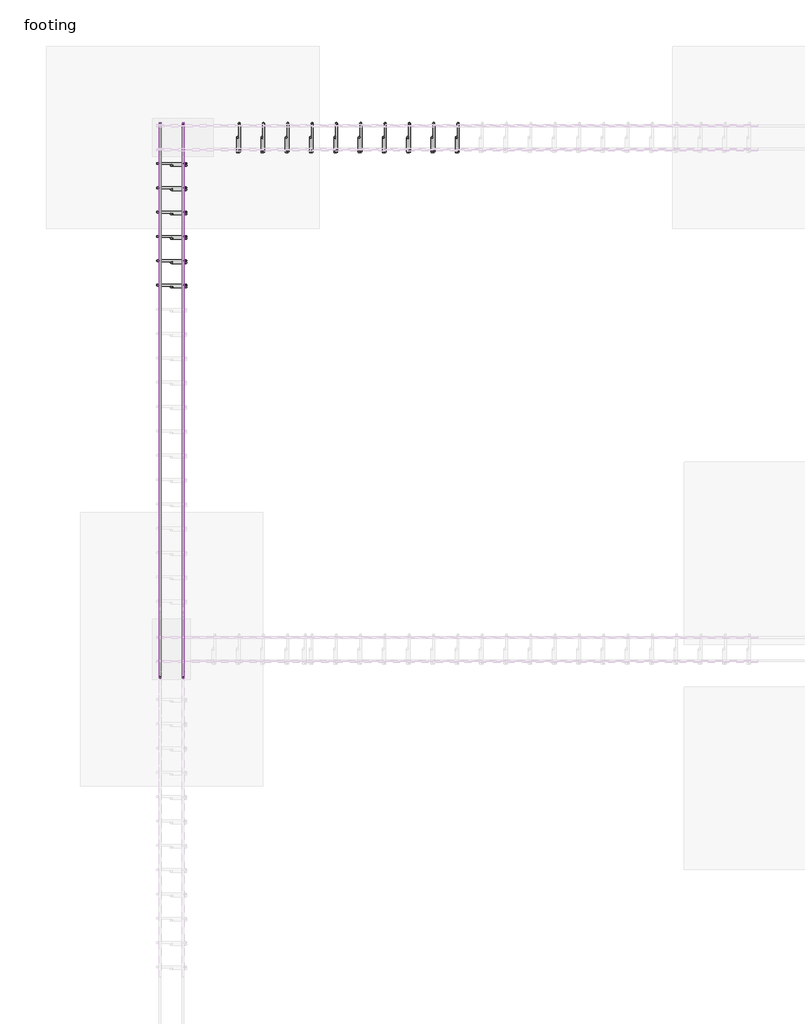
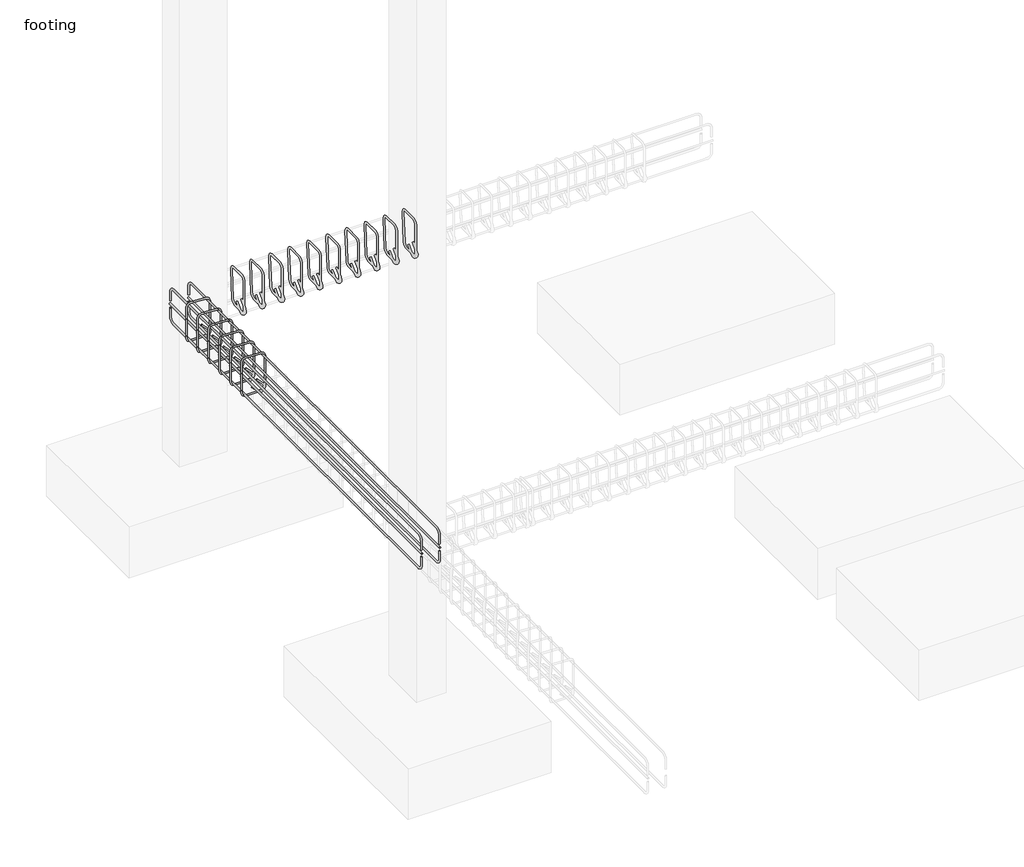
# One storey, part 16 of 21: 23 reinforcing bars.
"""IFC4 building model written with IfcOpenShell, lengths in millimetres."""

from ifc_helpers import new_model, si_unit, point, frame, origin, place, context, project, spatial, polyline, circle_curve, trimmed, segment, composite_curve, element, save
from ifc_brep_helpers import swept_disk

model = new_model("IFC4")

# Units and contexts
model_context = context("Model", 3, world=origin())
ifc_project = project(units=[si_unit("LENGTHUNIT", "METRE", prefix="MILLI")], contexts=[model_context])

# Site, building, storey
site = spatial("IfcSite", under=ifc_project)
building = spatial("IfcBuilding", under=site)
storey = spatial("IfcBuildingStorey", under=building, Name="footing", Elevation=-1524.0)

# Reinforcing bars
placement = place(None, origin())
element("IfcReinforcingBar", 1, at=placement, inside=storey, context=model_context, shape_type="SolidModel", body=[
    swept_disk(composite_curve([segment(polyline([(-11769.5883428, 10994.9387132, -310.8825168), (-11769.5883428, 10940.0737147, -365.7475153)]), True, "CONTINUOUS"), segment(trimmed(circle_curve(frame((-11769.5883428, 10917.6230744, -343.296875), z_axis=(-1.0, 0.0, 0.0), x_axis=(0.0, 22.450640299999577, -22.450640299999975)), 31.75), [point((-11769.5883428, 10940.0737147, -365.7475153))], [point((-11769.5883428, 10885.8730744, -343.296875))], True, "CARTESIAN"), True, "CONTINUOUS"), segment(polyline([(-11769.5883428, 10885.8730744, -343.296875), (-11769.5883428, 10885.8730744, -63.103125)]), True, "CONTINUOUS"), segment(trimmed(circle_curve(frame((-11769.5883428, 10917.6230744, -63.103125), z_axis=(-1.0, 0.0, 0.0), x_axis=(0.0, -31.75, 0.0)), 31.75), [point((-11769.5883428, 10885.8730744, -63.103125))], [point((-11769.5883428, 10917.6230744, -31.353125))], True, "CARTESIAN"), True, "CONTINUOUS"), segment(polyline([(-11769.5883428, 10917.6230744, -31.353125), (-11769.5883428, 11045.4168244, -31.353125)]), True, "CONTINUOUS"), segment(trimmed(circle_curve(frame((-11768.4159328, 11045.4168244, -63.0814712), z_axis=(-0.9993179916193466, 0.0, -0.03692629992126919), x_axis=(-1.1724099999992177, 0.0, 31.728346200000004)), 31.75), [point((-11769.5883428, 11045.4168244, -31.353125))], [point((-11768.4159328, 11077.1668244, -63.0814712))], True, "CARTESIAN"), True, "CONTINUOUS"), segment(polyline([(-11768.4159328, 11077.1668244, -63.0814712), (-11758.0607528, 11077.1668244, -343.3185288)]), True, "CONTINUOUS"), segment(trimmed(circle_curve(frame((-11758.0607528, 11045.4168244, -343.3185288), z_axis=(-0.9993179916193466, 0.0, -0.03692629992126919), x_axis=(0.0, 31.75, 0.0)), 31.75), [point((-11758.0607528, 11077.1668244, -343.3185288))], [point((-11756.8883428, 11045.4168244, -375.046875))], True, "CARTESIAN"), True, "CONTINUOUS"), segment(polyline([(-11756.8883428, 11045.4168244, -375.046875), (-11756.8883428, 10917.6230744, -375.046875)]), True, "CONTINUOUS"), segment(trimmed(circle_curve(frame((-11756.8883428, 10917.6230744, -343.296875), z_axis=(-1.0, 0.0, 0.0), x_axis=(0.0, 0.0, -31.75)), 31.75), [point((-11756.8883428, 10917.6230744, -375.046875))], [point((-11756.8883428, 10895.1724341, -320.8462347))], True, "CARTESIAN"), True, "CONTINUOUS"), segment(polyline([(-11756.8883428, 10895.1724341, -320.8462347), (-11756.8883428, 10950.0374326, -265.9812362)]), True, "CONTINUOUS")], self_intersect=False), 6.35),
])
element("IfcReinforcingBar", 2, at=placement, inside=storey, context=model_context, shape_type="SolidModel", body=[
    swept_disk(composite_curve([segment(polyline([(-11606.8883428, 10994.9387132, -310.8825168), (-11606.8883428, 10940.0737147, -365.7475153)]), True, "CONTINUOUS"), segment(trimmed(circle_curve(frame((-11606.8883428, 10917.6230744, -343.296875), z_axis=(-1.0, 0.0, 0.0), x_axis=(0.0, 22.450640299999577, -22.450640299999975)), 31.75), [point((-11606.8883428, 10940.0737147, -365.7475153))], [point((-11606.8883428, 10885.8730744, -343.296875))], True, "CARTESIAN"), True, "CONTINUOUS"), segment(polyline([(-11606.8883428, 10885.8730744, -343.296875), (-11606.8883428, 10885.8730744, -63.103125)]), True, "CONTINUOUS"), segment(trimmed(circle_curve(frame((-11606.8883428, 10917.6230744, -63.103125), z_axis=(-1.0, 0.0, 0.0), x_axis=(0.0, -31.75, 0.0)), 31.75), [point((-11606.8883428, 10885.8730744, -63.103125))], [point((-11606.8883428, 10917.6230744, -31.353125))], True, "CARTESIAN"), True, "CONTINUOUS"), segment(polyline([(-11606.8883428, 10917.6230744, -31.353125), (-11606.8883428, 11045.4168244, -31.353125)]), True, "CONTINUOUS"), segment(trimmed(circle_curve(frame((-11605.7159328, 11045.4168244, -63.0814712), z_axis=(-0.9993179916193466, 0.0, -0.03692629992126919), x_axis=(-1.1724100000010367, 0.0, 31.728346200000004)), 31.75), [point((-11606.8883428, 11045.4168244, -31.353125))], [point((-11605.7159328, 11077.1668244, -63.0814712))], True, "CARTESIAN"), True, "CONTINUOUS"), segment(polyline([(-11605.7159328, 11077.1668244, -63.0814712), (-11595.3607528, 11077.1668244, -343.3185288)]), True, "CONTINUOUS"), segment(trimmed(circle_curve(frame((-11595.3607528, 11045.4168244, -343.3185288), z_axis=(-0.9993179916193466, 0.0, -0.03692629992126919), x_axis=(0.0, 31.75, 0.0)), 31.75), [point((-11595.3607528, 11077.1668244, -343.3185288))], [point((-11594.1883428, 11045.4168244, -375.046875))], True, "CARTESIAN"), True, "CONTINUOUS"), segment(polyline([(-11594.1883428, 11045.4168244, -375.046875), (-11594.1883428, 10917.6230744, -375.046875)]), True, "CONTINUOUS"), segment(trimmed(circle_curve(frame((-11594.1883428, 10917.6230744, -343.296875), z_axis=(-1.0, 0.0, 0.0), x_axis=(0.0, 0.0, -31.75)), 31.75), [point((-11594.1883428, 10917.6230744, -375.046875))], [point((-11594.1883428, 10895.1724341, -320.8462347))], True, "CARTESIAN"), True, "CONTINUOUS"), segment(polyline([(-11594.1883428, 10895.1724341, -320.8462347), (-11594.1883428, 10950.0374326, -265.9812362)]), True, "CONTINUOUS")], self_intersect=False), 6.35),
])
element("IfcReinforcingBar", 3, at=placement, inside=storey, context=model_context, shape_type="SolidModel", body=[
    swept_disk(composite_curve([segment(polyline([(-11444.1883428, 10994.9387132, -310.8825168), (-11444.1883428, 10940.0737147, -365.7475153)]), True, "CONTINUOUS"), segment(trimmed(circle_curve(frame((-11444.1883428, 10917.6230744, -343.296875), z_axis=(-1.0, 0.0, 0.0), x_axis=(0.0, 22.450640299999577, -22.450640299999975)), 31.75), [point((-11444.1883428, 10940.0737147, -365.7475153))], [point((-11444.1883428, 10885.8730744, -343.296875))], True, "CARTESIAN"), True, "CONTINUOUS"), segment(polyline([(-11444.1883428, 10885.8730744, -343.296875), (-11444.1883428, 10885.8730744, -63.103125)]), True, "CONTINUOUS"), segment(trimmed(circle_curve(frame((-11444.1883428, 10917.6230744, -63.103125), z_axis=(-1.0, 0.0, 0.0), x_axis=(0.0, -31.75, 0.0)), 31.75), [point((-11444.1883428, 10885.8730744, -63.103125))], [point((-11444.1883428, 10917.6230744, -31.353125))], True, "CARTESIAN"), True, "CONTINUOUS"), segment(polyline([(-11444.1883428, 10917.6230744, -31.353125), (-11444.1883428, 11045.4168244, -31.353125)]), True, "CONTINUOUS"), segment(trimmed(circle_curve(frame((-11443.0159328, 11045.4168244, -63.0814712), z_axis=(-0.9993179916193466, 0.0, -0.03692629992126919), x_axis=(-1.1724099999992177, 0.0, 31.728346200000004)), 31.75), [point((-11444.1883428, 11045.4168244, -31.353125))], [point((-11443.0159328, 11077.1668244, -63.0814712))], True, "CARTESIAN"), True, "CONTINUOUS"), segment(polyline([(-11443.0159328, 11077.1668244, -63.0814712), (-11432.6607528, 11077.1668244, -343.3185288)]), True, "CONTINUOUS"), segment(trimmed(circle_curve(frame((-11432.6607528, 11045.4168244, -343.3185288), z_axis=(-0.9993179916193466, 0.0, -0.03692629992126919), x_axis=(0.0, 31.75, 0.0)), 31.75), [point((-11432.6607528, 11077.1668244, -343.3185288))], [point((-11431.4883428, 11045.4168244, -375.046875))], True, "CARTESIAN"), True, "CONTINUOUS"), segment(polyline([(-11431.4883428, 11045.4168244, -375.046875), (-11431.4883428, 10917.6230744, -375.046875)]), True, "CONTINUOUS"), segment(trimmed(circle_curve(frame((-11431.4883428, 10917.6230744, -343.296875), z_axis=(-1.0, 0.0, 0.0), x_axis=(0.0, 0.0, -31.75)), 31.75), [point((-11431.4883428, 10917.6230744, -375.046875))], [point((-11431.4883428, 10895.1724341, -320.8462347))], True, "CARTESIAN"), True, "CONTINUOUS"), segment(polyline([(-11431.4883428, 10895.1724341, -320.8462347), (-11431.4883428, 10950.0374326, -265.9812362)]), True, "CONTINUOUS")], self_intersect=False), 6.35),
])
element("IfcReinforcingBar", 4, at=placement, inside=storey, context=model_context, shape_type="SolidModel", body=[
    swept_disk(composite_curve([segment(polyline([(-11281.4883428, 10994.9387132, -310.8825168), (-11281.4883428, 10940.0737147, -365.7475153)]), True, "CONTINUOUS"), segment(trimmed(circle_curve(frame((-11281.4883428, 10917.6230744, -343.296875), z_axis=(-1.0, 0.0, 0.0), x_axis=(0.0, 22.450640299999577, -22.450640299999975)), 31.75), [point((-11281.4883428, 10940.0737147, -365.7475153))], [point((-11281.4883428, 10885.8730744, -343.296875))], True, "CARTESIAN"), True, "CONTINUOUS"), segment(polyline([(-11281.4883428, 10885.8730744, -343.296875), (-11281.4883428, 10885.8730744, -63.103125)]), True, "CONTINUOUS"), segment(trimmed(circle_curve(frame((-11281.4883428, 10917.6230744, -63.103125), z_axis=(-1.0, 0.0, 0.0), x_axis=(0.0, -31.75, 0.0)), 31.75), [point((-11281.4883428, 10885.8730744, -63.103125))], [point((-11281.4883428, 10917.6230744, -31.353125))], True, "CARTESIAN"), True, "CONTINUOUS"), segment(polyline([(-11281.4883428, 10917.6230744, -31.353125), (-11281.4883428, 11045.4168244, -31.353125)]), True, "CONTINUOUS"), segment(trimmed(circle_curve(frame((-11280.3159328, 11045.4168244, -63.0814712), z_axis=(-0.9993179916193466, 0.0, -0.03692629992126919), x_axis=(-1.1724099999992177, 0.0, 31.728346200000004)), 31.75), [point((-11281.4883428, 11045.4168244, -31.353125))], [point((-11280.3159328, 11077.1668244, -63.0814712))], True, "CARTESIAN"), True, "CONTINUOUS"), segment(polyline([(-11280.3159328, 11077.1668244, -63.0814712), (-11269.9607528, 11077.1668244, -343.3185288)]), True, "CONTINUOUS"), segment(trimmed(circle_curve(frame((-11269.9607528, 11045.4168244, -343.3185288), z_axis=(-0.9993179916193466, 0.0, -0.03692629992126919), x_axis=(0.0, 31.75, 0.0)), 31.75), [point((-11269.9607528, 11077.1668244, -343.3185288))], [point((-11268.7883428, 11045.4168244, -375.046875))], True, "CARTESIAN"), True, "CONTINUOUS"), segment(polyline([(-11268.7883428, 11045.4168244, -375.046875), (-11268.7883428, 10917.6230744, -375.046875)]), True, "CONTINUOUS"), segment(trimmed(circle_curve(frame((-11268.7883428, 10917.6230744, -343.296875), z_axis=(-1.0, 0.0, 0.0), x_axis=(0.0, 0.0, -31.75)), 31.75), [point((-11268.7883428, 10917.6230744, -375.046875))], [point((-11268.7883428, 10895.1724341, -320.8462347))], True, "CARTESIAN"), True, "CONTINUOUS"), segment(polyline([(-11268.7883428, 10895.1724341, -320.8462347), (-11268.7883428, 10950.0374326, -265.9812362)]), True, "CONTINUOUS")], self_intersect=False), 6.35),
])
element("IfcReinforcingBar", 5, at=placement, inside=storey, context=model_context, shape_type="SolidModel", body=[
    swept_disk(composite_curve([segment(polyline([(-11118.7883428, 10994.9387132, -310.8825168), (-11118.7883428, 10940.0737147, -365.7475153)]), True, "CONTINUOUS"), segment(trimmed(circle_curve(frame((-11118.7883428, 10917.6230744, -343.296875), z_axis=(-1.0, 0.0, 0.0), x_axis=(0.0, 22.450640299999577, -22.450640299999975)), 31.75), [point((-11118.7883428, 10940.0737147, -365.7475153))], [point((-11118.7883428, 10885.8730744, -343.296875))], True, "CARTESIAN"), True, "CONTINUOUS"), segment(polyline([(-11118.7883428, 10885.8730744, -343.296875), (-11118.7883428, 10885.8730744, -63.103125)]), True, "CONTINUOUS"), segment(trimmed(circle_curve(frame((-11118.7883428, 10917.6230744, -63.103125), z_axis=(-1.0, 0.0, 0.0), x_axis=(0.0, -31.75, 0.0)), 31.75), [point((-11118.7883428, 10885.8730744, -63.103125))], [point((-11118.7883428, 10917.6230744, -31.353125))], True, "CARTESIAN"), True, "CONTINUOUS"), segment(polyline([(-11118.7883428, 10917.6230744, -31.353125), (-11118.7883428, 11045.4168244, -31.353125)]), True, "CONTINUOUS"), segment(trimmed(circle_curve(frame((-11117.6159328, 11045.4168244, -63.0814712), z_axis=(-0.9993179916193466, 0.0, -0.03692629992126919), x_axis=(-1.1724100000010367, 0.0, 31.728346200000004)), 31.75), [point((-11118.7883428, 11045.4168244, -31.353125))], [point((-11117.6159328, 11077.1668244, -63.0814712))], True, "CARTESIAN"), True, "CONTINUOUS"), segment(polyline([(-11117.6159328, 11077.1668244, -63.0814712), (-11107.2607528, 11077.1668244, -343.3185288)]), True, "CONTINUOUS"), segment(trimmed(circle_curve(frame((-11107.2607528, 11045.4168244, -343.3185288), z_axis=(-0.9993179916193466, 0.0, -0.03692629992126919), x_axis=(0.0, 31.75, 0.0)), 31.75), [point((-11107.2607528, 11077.1668244, -343.3185288))], [point((-11106.0883428, 11045.4168244, -375.046875))], True, "CARTESIAN"), True, "CONTINUOUS"), segment(polyline([(-11106.0883428, 11045.4168244, -375.046875), (-11106.0883428, 10917.6230744, -375.046875)]), True, "CONTINUOUS"), segment(trimmed(circle_curve(frame((-11106.0883428, 10917.6230744, -343.296875), z_axis=(-1.0, 0.0, 0.0), x_axis=(0.0, 0.0, -31.75)), 31.75), [point((-11106.0883428, 10917.6230744, -375.046875))], [point((-11106.0883428, 10895.1724341, -320.8462347))], True, "CARTESIAN"), True, "CONTINUOUS"), segment(polyline([(-11106.0883428, 10895.1724341, -320.8462347), (-11106.0883428, 10950.0374326, -265.9812362)]), True, "CONTINUOUS")], self_intersect=False), 6.35),
])
element("IfcReinforcingBar", 6, at=placement, inside=storey, context=model_context, shape_type="SolidModel", body=[
    swept_disk(composite_curve([segment(polyline([(-10956.0883428, 10994.9387132, -310.8825168), (-10956.0883428, 10940.0737147, -365.7475153)]), True, "CONTINUOUS"), segment(trimmed(circle_curve(frame((-10956.0883428, 10917.6230744, -343.296875), z_axis=(-1.0, 0.0, 0.0), x_axis=(0.0, 22.450640299999577, -22.450640299999975)), 31.75), [point((-10956.0883428, 10940.0737147, -365.7475153))], [point((-10956.0883428, 10885.8730744, -343.296875))], True, "CARTESIAN"), True, "CONTINUOUS"), segment(polyline([(-10956.0883428, 10885.8730744, -343.296875), (-10956.0883428, 10885.8730744, -63.103125)]), True, "CONTINUOUS"), segment(trimmed(circle_curve(frame((-10956.0883428, 10917.6230744, -63.103125), z_axis=(-1.0, 0.0, 0.0), x_axis=(0.0, -31.75, 0.0)), 31.75), [point((-10956.0883428, 10885.8730744, -63.103125))], [point((-10956.0883428, 10917.6230744, -31.353125))], True, "CARTESIAN"), True, "CONTINUOUS"), segment(polyline([(-10956.0883428, 10917.6230744, -31.353125), (-10956.0883428, 11045.4168244, -31.353125)]), True, "CONTINUOUS"), segment(trimmed(circle_curve(frame((-10954.9159328, 11045.4168244, -63.0814712), z_axis=(-0.9993179916193466, 0.0, -0.03692629992126919), x_axis=(-1.1724099999992177, 0.0, 31.728346200000004)), 31.75), [point((-10956.0883428, 11045.4168244, -31.353125))], [point((-10954.9159328, 11077.1668244, -63.0814712))], True, "CARTESIAN"), True, "CONTINUOUS"), segment(polyline([(-10954.9159328, 11077.1668244, -63.0814712), (-10944.5607528, 11077.1668244, -343.3185288)]), True, "CONTINUOUS"), segment(trimmed(circle_curve(frame((-10944.5607528, 11045.4168244, -343.3185288), z_axis=(-0.9993179916193466, 0.0, -0.03692629992126919), x_axis=(0.0, 31.75, 0.0)), 31.75), [point((-10944.5607528, 11077.1668244, -343.3185288))], [point((-10943.3883428, 11045.4168244, -375.046875))], True, "CARTESIAN"), True, "CONTINUOUS"), segment(polyline([(-10943.3883428, 11045.4168244, -375.046875), (-10943.3883428, 10917.6230744, -375.046875)]), True, "CONTINUOUS"), segment(trimmed(circle_curve(frame((-10943.3883428, 10917.6230744, -343.296875), z_axis=(-1.0, 0.0, 0.0), x_axis=(0.0, 0.0, -31.75)), 31.75), [point((-10943.3883428, 10917.6230744, -375.046875))], [point((-10943.3883428, 10895.1724341, -320.8462347))], True, "CARTESIAN"), True, "CONTINUOUS"), segment(polyline([(-10943.3883428, 10895.1724341, -320.8462347), (-10943.3883428, 10950.0374326, -265.9812362)]), True, "CONTINUOUS")], self_intersect=False), 6.35),
])
element("IfcReinforcingBar", 7, at=placement, inside=storey, context=model_context, shape_type="SolidModel", body=[
    swept_disk(composite_curve([segment(polyline([(-10793.3883428, 10994.9387132, -310.8825168), (-10793.3883428, 10940.0737147, -365.7475153)]), True, "CONTINUOUS"), segment(trimmed(circle_curve(frame((-10793.3883428, 10917.6230744, -343.296875), z_axis=(-1.0, 0.0, 0.0), x_axis=(0.0, 22.450640299999577, -22.450640299999975)), 31.75), [point((-10793.3883428, 10940.0737147, -365.7475153))], [point((-10793.3883428, 10885.8730744, -343.296875))], True, "CARTESIAN"), True, "CONTINUOUS"), segment(polyline([(-10793.3883428, 10885.8730744, -343.296875), (-10793.3883428, 10885.8730744, -63.103125)]), True, "CONTINUOUS"), segment(trimmed(circle_curve(frame((-10793.3883428, 10917.6230744, -63.103125), z_axis=(-1.0, 0.0, 0.0), x_axis=(0.0, -31.75, 0.0)), 31.75), [point((-10793.3883428, 10885.8730744, -63.103125))], [point((-10793.3883428, 10917.6230744, -31.353125))], True, "CARTESIAN"), True, "CONTINUOUS"), segment(polyline([(-10793.3883428, 10917.6230744, -31.353125), (-10793.3883428, 11045.4168244, -31.353125)]), True, "CONTINUOUS"), segment(trimmed(circle_curve(frame((-10792.2159328, 11045.4168244, -63.0814712), z_axis=(-0.9993179916193466, 0.0, -0.03692629992126919), x_axis=(-1.1724100000010367, 0.0, 31.728346200000004)), 31.75), [point((-10793.3883428, 11045.4168244, -31.353125))], [point((-10792.2159328, 11077.1668244, -63.0814712))], True, "CARTESIAN"), True, "CONTINUOUS"), segment(polyline([(-10792.2159328, 11077.1668244, -63.0814712), (-10781.8607528, 11077.1668244, -343.3185288)]), True, "CONTINUOUS"), segment(trimmed(circle_curve(frame((-10781.8607528, 11045.4168244, -343.3185288), z_axis=(-0.9993179916193466, 0.0, -0.03692629992126919), x_axis=(0.0, 31.75, 0.0)), 31.75), [point((-10781.8607528, 11077.1668244, -343.3185288))], [point((-10780.6883428, 11045.4168244, -375.046875))], True, "CARTESIAN"), True, "CONTINUOUS"), segment(polyline([(-10780.6883428, 11045.4168244, -375.046875), (-10780.6883428, 10917.6230744, -375.046875)]), True, "CONTINUOUS"), segment(trimmed(circle_curve(frame((-10780.6883428, 10917.6230744, -343.296875), z_axis=(-1.0, 0.0, 0.0), x_axis=(0.0, 0.0, -31.75)), 31.75), [point((-10780.6883428, 10917.6230744, -375.046875))], [point((-10780.6883428, 10895.1724341, -320.8462347))], True, "CARTESIAN"), True, "CONTINUOUS"), segment(polyline([(-10780.6883428, 10895.1724341, -320.8462347), (-10780.6883428, 10950.0374326, -265.9812362)]), True, "CONTINUOUS")], self_intersect=False), 6.35),
])
element("IfcReinforcingBar", 8, at=placement, inside=storey, context=model_context, shape_type="SolidModel", body=[
    swept_disk(composite_curve([segment(polyline([(-10630.6883428, 10994.9387132, -310.8825168), (-10630.6883428, 10940.0737147, -365.7475153)]), True, "CONTINUOUS"), segment(trimmed(circle_curve(frame((-10630.6883428, 10917.6230744, -343.296875), z_axis=(-1.0, 0.0, 0.0), x_axis=(0.0, 22.450640299999577, -22.450640299999975)), 31.75), [point((-10630.6883428, 10940.0737147, -365.7475153))], [point((-10630.6883428, 10885.8730744, -343.296875))], True, "CARTESIAN"), True, "CONTINUOUS"), segment(polyline([(-10630.6883428, 10885.8730744, -343.296875), (-10630.6883428, 10885.8730744, -63.103125)]), True, "CONTINUOUS"), segment(trimmed(circle_curve(frame((-10630.6883428, 10917.6230744, -63.103125), z_axis=(-1.0, 0.0, 0.0), x_axis=(0.0, -31.75, 0.0)), 31.75), [point((-10630.6883428, 10885.8730744, -63.103125))], [point((-10630.6883428, 10917.6230744, -31.353125))], True, "CARTESIAN"), True, "CONTINUOUS"), segment(polyline([(-10630.6883428, 10917.6230744, -31.353125), (-10630.6883428, 11045.4168244, -31.353125)]), True, "CONTINUOUS"), segment(trimmed(circle_curve(frame((-10629.5159328, 11045.4168244, -63.0814712), z_axis=(-0.9993179916193466, 0.0, -0.03692629992126919), x_axis=(-1.1724099999992177, 0.0, 31.728346200000004)), 31.75), [point((-10630.6883428, 11045.4168244, -31.353125))], [point((-10629.5159328, 11077.1668244, -63.0814712))], True, "CARTESIAN"), True, "CONTINUOUS"), segment(polyline([(-10629.5159328, 11077.1668244, -63.0814712), (-10619.1607528, 11077.1668244, -343.3185288)]), True, "CONTINUOUS"), segment(trimmed(circle_curve(frame((-10619.1607528, 11045.4168244, -343.3185288), z_axis=(-0.9993179916193466, 0.0, -0.03692629992126919), x_axis=(0.0, 31.75, 0.0)), 31.75), [point((-10619.1607528, 11077.1668244, -343.3185288))], [point((-10617.9883428, 11045.4168244, -375.046875))], True, "CARTESIAN"), True, "CONTINUOUS"), segment(polyline([(-10617.9883428, 11045.4168244, -375.046875), (-10617.9883428, 10917.6230744, -375.046875)]), True, "CONTINUOUS"), segment(trimmed(circle_curve(frame((-10617.9883428, 10917.6230744, -343.296875), z_axis=(-1.0, 0.0, 0.0), x_axis=(0.0, 0.0, -31.75)), 31.75), [point((-10617.9883428, 10917.6230744, -375.046875))], [point((-10617.9883428, 10895.1724341, -320.8462347))], True, "CARTESIAN"), True, "CONTINUOUS"), segment(polyline([(-10617.9883428, 10895.1724341, -320.8462347), (-10617.9883428, 10950.0374326, -265.9812362)]), True, "CONTINUOUS")], self_intersect=False), 6.35),
])
element("IfcReinforcingBar", 9, at=placement, inside=storey, context=model_context, shape_type="SolidModel", body=[
    swept_disk(composite_curve([segment(polyline([(-10467.9883428, 10994.9387132, -310.8825168), (-10467.9883428, 10940.0737147, -365.7475153)]), True, "CONTINUOUS"), segment(trimmed(circle_curve(frame((-10467.9883428, 10917.6230744, -343.296875), z_axis=(-1.0, 0.0, 0.0), x_axis=(0.0, 22.450640299999577, -22.450640299999975)), 31.75), [point((-10467.9883428, 10940.0737147, -365.7475153))], [point((-10467.9883428, 10885.8730744, -343.296875))], True, "CARTESIAN"), True, "CONTINUOUS"), segment(polyline([(-10467.9883428, 10885.8730744, -343.296875), (-10467.9883428, 10885.8730744, -63.103125)]), True, "CONTINUOUS"), segment(trimmed(circle_curve(frame((-10467.9883428, 10917.6230744, -63.103125), z_axis=(-1.0, 0.0, 0.0), x_axis=(0.0, -31.75, 0.0)), 31.75), [point((-10467.9883428, 10885.8730744, -63.103125))], [point((-10467.9883428, 10917.6230744, -31.353125))], True, "CARTESIAN"), True, "CONTINUOUS"), segment(polyline([(-10467.9883428, 10917.6230744, -31.353125), (-10467.9883428, 11045.4168244, -31.353125)]), True, "CONTINUOUS"), segment(trimmed(circle_curve(frame((-10466.8159328, 11045.4168244, -63.0814712), z_axis=(-0.9993179916193466, 0.0, -0.03692629992126919), x_axis=(-1.1724099999992177, 0.0, 31.728346200000004)), 31.75), [point((-10467.9883428, 11045.4168244, -31.353125))], [point((-10466.8159328, 11077.1668244, -63.0814712))], True, "CARTESIAN"), True, "CONTINUOUS"), segment(polyline([(-10466.8159328, 11077.1668244, -63.0814712), (-10456.4607528, 11077.1668244, -343.3185288)]), True, "CONTINUOUS"), segment(trimmed(circle_curve(frame((-10456.4607528, 11045.4168244, -343.3185288), z_axis=(-0.9993179916193466, 0.0, -0.03692629992126919), x_axis=(0.0, 31.75, 0.0)), 31.75), [point((-10456.4607528, 11077.1668244, -343.3185288))], [point((-10455.2883428, 11045.4168244, -375.046875))], True, "CARTESIAN"), True, "CONTINUOUS"), segment(polyline([(-10455.2883428, 11045.4168244, -375.046875), (-10455.2883428, 10917.6230744, -375.046875)]), True, "CONTINUOUS"), segment(trimmed(circle_curve(frame((-10455.2883428, 10917.6230744, -343.296875), z_axis=(-1.0, 0.0, 0.0), x_axis=(0.0, 0.0, -31.75)), 31.75), [point((-10455.2883428, 10917.6230744, -375.046875))], [point((-10455.2883428, 10895.1724341, -320.8462347))], True, "CARTESIAN"), True, "CONTINUOUS"), segment(polyline([(-10455.2883428, 10895.1724341, -320.8462347), (-10455.2883428, 10950.0374326, -265.9812362)]), True, "CONTINUOUS")], self_intersect=False), 6.35),
])
element("IfcReinforcingBar", 10, at=placement, inside=storey, context=model_context, shape_type="SolidModel", body=[
    swept_disk(composite_curve([segment(polyline([(-10305.2883428, 10994.9387132, -310.8825168), (-10305.2883428, 10940.0737147, -365.7475153)]), True, "CONTINUOUS"), segment(trimmed(circle_curve(frame((-10305.2883428, 10917.6230744, -343.296875), z_axis=(-1.0, 0.0, 0.0), x_axis=(0.0, 22.450640299999577, -22.450640299999975)), 31.75), [point((-10305.2883428, 10940.0737147, -365.7475153))], [point((-10305.2883428, 10885.8730744, -343.296875))], True, "CARTESIAN"), True, "CONTINUOUS"), segment(polyline([(-10305.2883428, 10885.8730744, -343.296875), (-10305.2883428, 10885.8730744, -63.103125)]), True, "CONTINUOUS"), segment(trimmed(circle_curve(frame((-10305.2883428, 10917.6230744, -63.103125), z_axis=(-1.0, 0.0, 0.0), x_axis=(0.0, -31.75, 0.0)), 31.75), [point((-10305.2883428, 10885.8730744, -63.103125))], [point((-10305.2883428, 10917.6230744, -31.353125))], True, "CARTESIAN"), True, "CONTINUOUS"), segment(polyline([(-10305.2883428, 10917.6230744, -31.353125), (-10305.2883428, 11045.4168244, -31.353125)]), True, "CONTINUOUS"), segment(trimmed(circle_curve(frame((-10304.1159328, 11045.4168244, -63.0814712), z_axis=(-0.9993179916193466, 0.0, -0.03692629992126919), x_axis=(-1.1724100000010367, 0.0, 31.728346200000004)), 31.75), [point((-10305.2883428, 11045.4168244, -31.353125))], [point((-10304.1159328, 11077.1668244, -63.0814712))], True, "CARTESIAN"), True, "CONTINUOUS"), segment(polyline([(-10304.1159328, 11077.1668244, -63.0814712), (-10293.7607528, 11077.1668244, -343.3185288)]), True, "CONTINUOUS"), segment(trimmed(circle_curve(frame((-10293.7607528, 11045.4168244, -343.3185288), z_axis=(-0.9993179916193466, 0.0, -0.03692629992126919), x_axis=(0.0, 31.75, 0.0)), 31.75), [point((-10293.7607528, 11077.1668244, -343.3185288))], [point((-10292.5883428, 11045.4168244, -375.046875))], True, "CARTESIAN"), True, "CONTINUOUS"), segment(polyline([(-10292.5883428, 11045.4168244, -375.046875), (-10292.5883428, 10917.6230744, -375.046875)]), True, "CONTINUOUS"), segment(trimmed(circle_curve(frame((-10292.5883428, 10917.6230744, -343.296875), z_axis=(-1.0, 0.0, 0.0), x_axis=(0.0, 0.0, -31.75)), 31.75), [point((-10292.5883428, 10917.6230744, -375.046875))], [point((-10292.5883428, 10895.1724341, -320.8462347))], True, "CARTESIAN"), True, "CONTINUOUS"), segment(polyline([(-10292.5883428, 10895.1724341, -320.8462347), (-10292.5883428, 10950.0374326, -265.9812362)]), True, "CONTINUOUS")], self_intersect=False), 6.35),
])
element("IfcReinforcingBar", 11, at=placement, inside=storey, context=model_context, shape_type="SolidModel", body=[
    swept_disk(composite_curve([segment(polyline([(-12178.1165254, 9995.2456073, -265.9812362), (-12123.251527, 9995.2456073, -320.8462347)]), True, "CONTINUOUS"), segment(trimmed(circle_curve(frame((-12145.7021673, 9995.2456073, -343.296875), z_axis=(0.0, 1.0, 0.0), x_axis=(22.450640299999577, 0.0, 22.450640299999975)), 31.75), [point((-12123.251527, 9995.2456073, -320.8462347))], [point((-12145.7021673, 9995.2456073, -375.046875))], True, "CARTESIAN"), True, "CONTINUOUS"), segment(polyline([(-12145.7021673, 9995.2456073, -375.046875), (-12273.4959173, 9995.2456073, -375.046875)]), True, "CONTINUOUS"), segment(trimmed(circle_curve(frame((-12273.4959173, 9995.2456073, -343.296875), z_axis=(0.0, 1.0, 0.0), x_axis=(0.0, 0.0, -31.75)), 31.75), [point((-12273.4959173, 9995.2456073, -375.046875))], [point((-12305.2459173, 9995.2456073, -343.296875))], True, "CARTESIAN"), True, "CONTINUOUS"), segment(polyline([(-12305.2459173, 9995.2456073, -343.296875), (-12305.2459173, 9995.2456073, -63.103125)]), True, "CONTINUOUS"), segment(trimmed(circle_curve(frame((-12273.565658, 9993.1423536, -63.103125), z_axis=(0.0662442117686417, 0.9978034397651431, 0.0), x_axis=(-31.680259300001126, 2.103253699999186, 0.0)), 31.75), [point((-12305.2459173, 9995.2456073, -63.103125))], [point((-12273.565658, 9993.1423536, -31.353125))], True, "CARTESIAN"), True, "CONTINUOUS"), segment(polyline([(-12273.565658, 9993.1423536, -31.353125), (-12145.6324265, 9984.648861, -31.353125)]), True, "CONTINUOUS"), segment(trimmed(circle_curve(frame((-12145.6324265, 9984.648861, -63.103125), z_axis=(0.06624421176864169, 0.997803439765143, 0.0), x_axis=(0.0, 0.0, 31.75)), 31.75), [point((-12145.6324265, 9984.648861, -31.353125))], [point((-12113.9521673, 9982.5456073, -63.103125))], True, "CARTESIAN"), True, "CONTINUOUS"), segment(polyline([(-12113.9521673, 9982.5456073, -63.103125), (-12113.9521673, 9982.5456073, -343.296875)]), True, "CONTINUOUS"), segment(trimmed(circle_curve(frame((-12145.7021673, 9982.5456073, -343.296875), z_axis=(0.0, 1.0, 0.0), x_axis=(31.75, 0.0, 0.0)), 31.75), [point((-12113.9521673, 9982.5456073, -343.296875))], [point((-12168.1528076, 9982.5456073, -365.7475153))], True, "CARTESIAN"), True, "CONTINUOUS"), segment(polyline([(-12168.1528076, 9982.5456073, -365.7475153), (-12223.017806, 9982.5456073, -310.8825168)]), True, "CONTINUOUS")], self_intersect=False), 6.35),
])
element("IfcReinforcingBar", 12, at=placement, inside=storey, context=model_context, shape_type="SolidModel", body=[
    swept_disk(composite_curve([segment(polyline([(-12178.1165254, 10157.9456073, -265.9812362), (-12123.251527, 10157.9456073, -320.8462347)]), True, "CONTINUOUS"), segment(trimmed(circle_curve(frame((-12145.7021673, 10157.9456073, -343.296875), z_axis=(0.0, 1.0, 0.0), x_axis=(22.450640299999577, 0.0, 22.450640299999975)), 31.75), [point((-12123.251527, 10157.9456073, -320.8462347))], [point((-12145.7021673, 10157.9456073, -375.046875))], True, "CARTESIAN"), True, "CONTINUOUS"), segment(polyline([(-12145.7021673, 10157.9456073, -375.046875), (-12273.4959173, 10157.9456073, -375.046875)]), True, "CONTINUOUS"), segment(trimmed(circle_curve(frame((-12273.4959173, 10157.9456073, -343.296875), z_axis=(0.0, 1.0, 0.0), x_axis=(0.0, 0.0, -31.75)), 31.75), [point((-12273.4959173, 10157.9456073, -375.046875))], [point((-12305.2459173, 10157.9456073, -343.296875))], True, "CARTESIAN"), True, "CONTINUOUS"), segment(polyline([(-12305.2459173, 10157.9456073, -343.296875), (-12305.2459173, 10157.9456073, -63.103125)]), True, "CONTINUOUS"), segment(trimmed(circle_curve(frame((-12273.565658, 10155.8423536, -63.103125), z_axis=(0.0662442117686417, 0.9978034397651431, 0.0), x_axis=(-31.680259300001126, 2.103253700001005, 0.0)), 31.75), [point((-12305.2459173, 10157.9456073, -63.103125))], [point((-12273.565658, 10155.8423536, -31.353125))], True, "CARTESIAN"), True, "CONTINUOUS"), segment(polyline([(-12273.565658, 10155.8423536, -31.353125), (-12145.6324265, 10147.348861, -31.353125)]), True, "CONTINUOUS"), segment(trimmed(circle_curve(frame((-12145.6324265, 10147.348861, -63.103125), z_axis=(0.06624421176864169, 0.997803439765143, 0.0), x_axis=(0.0, 0.0, 31.75)), 31.75), [point((-12145.6324265, 10147.348861, -31.353125))], [point((-12113.9521673, 10145.2456073, -63.103125))], True, "CARTESIAN"), True, "CONTINUOUS"), segment(polyline([(-12113.9521673, 10145.2456073, -63.103125), (-12113.9521673, 10145.2456073, -343.296875)]), True, "CONTINUOUS"), segment(trimmed(circle_curve(frame((-12145.7021673, 10145.2456073, -343.296875), z_axis=(0.0, 1.0, 0.0), x_axis=(31.75, 0.0, 0.0)), 31.75), [point((-12113.9521673, 10145.2456073, -343.296875))], [point((-12168.1528076, 10145.2456073, -365.7475153))], True, "CARTESIAN"), True, "CONTINUOUS"), segment(polyline([(-12168.1528076, 10145.2456073, -365.7475153), (-12223.017806, 10145.2456073, -310.8825168)]), True, "CONTINUOUS")], self_intersect=False), 6.35),
])
element("IfcReinforcingBar", 13, at=placement, inside=storey, context=model_context, shape_type="SolidModel", body=[
    swept_disk(composite_curve([segment(polyline([(-12178.1165254, 10320.6456073, -265.9812362), (-12123.251527, 10320.6456073, -320.8462347)]), True, "CONTINUOUS"), segment(trimmed(circle_curve(frame((-12145.7021673, 10320.6456073, -343.296875), z_axis=(0.0, 1.0, 0.0), x_axis=(22.450640299999577, 0.0, 22.450640299999975)), 31.75), [point((-12123.251527, 10320.6456073, -320.8462347))], [point((-12145.7021673, 10320.6456073, -375.046875))], True, "CARTESIAN"), True, "CONTINUOUS"), segment(polyline([(-12145.7021673, 10320.6456073, -375.046875), (-12273.4959173, 10320.6456073, -375.046875)]), True, "CONTINUOUS"), segment(trimmed(circle_curve(frame((-12273.4959173, 10320.6456073, -343.296875), z_axis=(0.0, 1.0, 0.0), x_axis=(0.0, 0.0, -31.75)), 31.75), [point((-12273.4959173, 10320.6456073, -375.046875))], [point((-12305.2459173, 10320.6456073, -343.296875))], True, "CARTESIAN"), True, "CONTINUOUS"), segment(polyline([(-12305.2459173, 10320.6456073, -343.296875), (-12305.2459173, 10320.6456073, -63.103125)]), True, "CONTINUOUS"), segment(trimmed(circle_curve(frame((-12273.565658, 10318.5423536, -63.103125), z_axis=(0.0662442117686417, 0.9978034397651431, 0.0), x_axis=(-31.680259300001126, 2.103253700001005, 0.0)), 31.75), [point((-12305.2459173, 10320.6456073, -63.103125))], [point((-12273.565658, 10318.5423536, -31.353125))], True, "CARTESIAN"), True, "CONTINUOUS"), segment(polyline([(-12273.565658, 10318.5423536, -31.353125), (-12145.6324265, 10310.048861, -31.353125)]), True, "CONTINUOUS"), segment(trimmed(circle_curve(frame((-12145.6324265, 10310.048861, -63.103125), z_axis=(0.06624421176864169, 0.997803439765143, 0.0), x_axis=(0.0, 0.0, 31.75)), 31.75), [point((-12145.6324265, 10310.048861, -31.353125))], [point((-12113.9521673, 10307.9456073, -63.103125))], True, "CARTESIAN"), True, "CONTINUOUS"), segment(polyline([(-12113.9521673, 10307.9456073, -63.103125), (-12113.9521673, 10307.9456073, -343.296875)]), True, "CONTINUOUS"), segment(trimmed(circle_curve(frame((-12145.7021673, 10307.9456073, -343.296875), z_axis=(0.0, 1.0, 0.0), x_axis=(31.75, 0.0, 0.0)), 31.75), [point((-12113.9521673, 10307.9456073, -343.296875))], [point((-12168.1528076, 10307.9456073, -365.7475153))], True, "CARTESIAN"), True, "CONTINUOUS"), segment(polyline([(-12168.1528076, 10307.9456073, -365.7475153), (-12223.017806, 10307.9456073, -310.8825168)]), True, "CONTINUOUS")], self_intersect=False), 6.35),
])
element("IfcReinforcingBar", 14, at=placement, inside=storey, context=model_context, shape_type="SolidModel", body=[
    swept_disk(composite_curve([segment(polyline([(-12178.1165254, 10483.3456073, -265.9812362), (-12123.251527, 10483.3456073, -320.8462347)]), True, "CONTINUOUS"), segment(trimmed(circle_curve(frame((-12145.7021673, 10483.3456073, -343.296875), z_axis=(0.0, 1.0, 0.0), x_axis=(22.450640299999577, 0.0, 22.450640299999975)), 31.75), [point((-12123.251527, 10483.3456073, -320.8462347))], [point((-12145.7021673, 10483.3456073, -375.046875))], True, "CARTESIAN"), True, "CONTINUOUS"), segment(polyline([(-12145.7021673, 10483.3456073, -375.046875), (-12273.4959173, 10483.3456073, -375.046875)]), True, "CONTINUOUS"), segment(trimmed(circle_curve(frame((-12273.4959173, 10483.3456073, -343.296875), z_axis=(0.0, 1.0, 0.0), x_axis=(0.0, 0.0, -31.75)), 31.75), [point((-12273.4959173, 10483.3456073, -375.046875))], [point((-12305.2459173, 10483.3456073, -343.296875))], True, "CARTESIAN"), True, "CONTINUOUS"), segment(polyline([(-12305.2459173, 10483.3456073, -343.296875), (-12305.2459173, 10483.3456073, -63.103125)]), True, "CONTINUOUS"), segment(trimmed(circle_curve(frame((-12273.565658, 10481.2423536, -63.103125), z_axis=(0.0662442117686417, 0.9978034397651431, 0.0), x_axis=(-31.680259300001126, 2.103253699999186, 0.0)), 31.75), [point((-12305.2459173, 10483.3456073, -63.103125))], [point((-12273.565658, 10481.2423536, -31.353125))], True, "CARTESIAN"), True, "CONTINUOUS"), segment(polyline([(-12273.565658, 10481.2423536, -31.353125), (-12145.6324265, 10472.748861, -31.353125)]), True, "CONTINUOUS"), segment(trimmed(circle_curve(frame((-12145.6324265, 10472.748861, -63.103125), z_axis=(0.06624421176864169, 0.997803439765143, 0.0), x_axis=(0.0, 0.0, 31.75)), 31.75), [point((-12145.6324265, 10472.748861, -31.353125))], [point((-12113.9521673, 10470.6456073, -63.103125))], True, "CARTESIAN"), True, "CONTINUOUS"), segment(polyline([(-12113.9521673, 10470.6456073, -63.103125), (-12113.9521673, 10470.6456073, -343.296875)]), True, "CONTINUOUS"), segment(trimmed(circle_curve(frame((-12145.7021673, 10470.6456073, -343.296875), z_axis=(0.0, 1.0, 0.0), x_axis=(31.75, 0.0, 0.0)), 31.75), [point((-12113.9521673, 10470.6456073, -343.296875))], [point((-12168.1528076, 10470.6456073, -365.7475153))], True, "CARTESIAN"), True, "CONTINUOUS"), segment(polyline([(-12168.1528076, 10470.6456073, -365.7475153), (-12223.017806, 10470.6456073, -310.8825168)]), True, "CONTINUOUS")], self_intersect=False), 6.35),
])
element("IfcReinforcingBar", 15, at=placement, inside=storey, context=model_context, shape_type="SolidModel", body=[
    swept_disk(composite_curve([segment(polyline([(-12178.1165254, 10646.0456073, -265.9812362), (-12123.251527, 10646.0456073, -320.8462347)]), True, "CONTINUOUS"), segment(trimmed(circle_curve(frame((-12145.7021673, 10646.0456073, -343.296875), z_axis=(0.0, 1.0, 0.0), x_axis=(22.450640299999577, 0.0, 22.450640299999975)), 31.75), [point((-12123.251527, 10646.0456073, -320.8462347))], [point((-12145.7021673, 10646.0456073, -375.046875))], True, "CARTESIAN"), True, "CONTINUOUS"), segment(polyline([(-12145.7021673, 10646.0456073, -375.046875), (-12273.4959173, 10646.0456073, -375.046875)]), True, "CONTINUOUS"), segment(trimmed(circle_curve(frame((-12273.4959173, 10646.0456073, -343.296875), z_axis=(0.0, 1.0, 0.0), x_axis=(0.0, 0.0, -31.75)), 31.75), [point((-12273.4959173, 10646.0456073, -375.046875))], [point((-12305.2459173, 10646.0456073, -343.296875))], True, "CARTESIAN"), True, "CONTINUOUS"), segment(polyline([(-12305.2459173, 10646.0456073, -343.296875), (-12305.2459173, 10646.0456073, -63.103125)]), True, "CONTINUOUS"), segment(trimmed(circle_curve(frame((-12273.565658, 10643.9423536, -63.103125), z_axis=(0.0662442117686417, 0.9978034397651431, 0.0), x_axis=(-31.680259300001126, 2.103253700001005, 0.0)), 31.75), [point((-12305.2459173, 10646.0456073, -63.103125))], [point((-12273.565658, 10643.9423536, -31.353125))], True, "CARTESIAN"), True, "CONTINUOUS"), segment(polyline([(-12273.565658, 10643.9423536, -31.353125), (-12145.6324265, 10635.448861, -31.353125)]), True, "CONTINUOUS"), segment(trimmed(circle_curve(frame((-12145.6324265, 10635.448861, -63.103125), z_axis=(0.06624421176864169, 0.997803439765143, 0.0), x_axis=(0.0, 0.0, 31.75)), 31.75), [point((-12145.6324265, 10635.448861, -31.353125))], [point((-12113.9521673, 10633.3456073, -63.103125))], True, "CARTESIAN"), True, "CONTINUOUS"), segment(polyline([(-12113.9521673, 10633.3456073, -63.103125), (-12113.9521673, 10633.3456073, -343.296875)]), True, "CONTINUOUS"), segment(trimmed(circle_curve(frame((-12145.7021673, 10633.3456073, -343.296875), z_axis=(0.0, 1.0, 0.0), x_axis=(31.75, 0.0, 0.0)), 31.75), [point((-12113.9521673, 10633.3456073, -343.296875))], [point((-12168.1528076, 10633.3456073, -365.7475153))], True, "CARTESIAN"), True, "CONTINUOUS"), segment(polyline([(-12168.1528076, 10633.3456073, -365.7475153), (-12223.017806, 10633.3456073, -310.8825168)]), True, "CONTINUOUS")], self_intersect=False), 6.35),
])
element("IfcReinforcingBar", 16, at=placement, inside=storey, context=model_context, shape_type="SolidModel", body=[
    swept_disk(composite_curve([segment(polyline([(-12178.1165254, 10808.7456073, -265.9812362), (-12123.251527, 10808.7456073, -320.8462347)]), True, "CONTINUOUS"), segment(trimmed(circle_curve(frame((-12145.7021673, 10808.7456073, -343.296875), z_axis=(0.0, 1.0, 0.0), x_axis=(22.450640299999577, 0.0, 22.450640299999975)), 31.75), [point((-12123.251527, 10808.7456073, -320.8462347))], [point((-12145.7021673, 10808.7456073, -375.046875))], True, "CARTESIAN"), True, "CONTINUOUS"), segment(polyline([(-12145.7021673, 10808.7456073, -375.046875), (-12273.4959173, 10808.7456073, -375.046875)]), True, "CONTINUOUS"), segment(trimmed(circle_curve(frame((-12273.4959173, 10808.7456073, -343.296875), z_axis=(0.0, 1.0, 0.0), x_axis=(0.0, 0.0, -31.75)), 31.75), [point((-12273.4959173, 10808.7456073, -375.046875))], [point((-12305.2459173, 10808.7456073, -343.296875))], True, "CARTESIAN"), True, "CONTINUOUS"), segment(polyline([(-12305.2459173, 10808.7456073, -343.296875), (-12305.2459173, 10808.7456073, -63.103125)]), True, "CONTINUOUS"), segment(trimmed(circle_curve(frame((-12273.565658, 10806.6423536, -63.103125), z_axis=(0.0662442117686417, 0.9978034397651431, 0.0), x_axis=(-31.680259300001126, 2.103253699999186, 0.0)), 31.75), [point((-12305.2459173, 10808.7456073, -63.103125))], [point((-12273.565658, 10806.6423536, -31.353125))], True, "CARTESIAN"), True, "CONTINUOUS"), segment(polyline([(-12273.565658, 10806.6423536, -31.353125), (-12145.6324265, 10798.148861, -31.353125)]), True, "CONTINUOUS"), segment(trimmed(circle_curve(frame((-12145.6324265, 10798.148861, -63.103125), z_axis=(0.06624421176864169, 0.997803439765143, 0.0), x_axis=(0.0, 0.0, 31.75)), 31.75), [point((-12145.6324265, 10798.148861, -31.353125))], [point((-12113.9521673, 10796.0456073, -63.103125))], True, "CARTESIAN"), True, "CONTINUOUS"), segment(polyline([(-12113.9521673, 10796.0456073, -63.103125), (-12113.9521673, 10796.0456073, -343.296875)]), True, "CONTINUOUS"), segment(trimmed(circle_curve(frame((-12145.7021673, 10796.0456073, -343.296875), z_axis=(0.0, 1.0, 0.0), x_axis=(31.75, 0.0, 0.0)), 31.75), [point((-12113.9521673, 10796.0456073, -343.296875))], [point((-12168.1528076, 10796.0456073, -365.7475153))], True, "CARTESIAN"), True, "CONTINUOUS"), segment(polyline([(-12168.1528076, 10796.0456073, -365.7475153), (-12223.017806, 10796.0456073, -310.8825168)]), True, "CONTINUOUS")], self_intersect=False), 6.35),
])
element("IfcReinforcingBar", 17, at=placement, inside=storey, context=model_context, shape_type="SolidModel", body=[
    swept_disk(composite_curve([segment(polyline([(-12132.2317831, 7371.1859344, -170.2827408), (-12132.2317831, 7371.1859344, -94.0827408)]), True, "CONTINUOUS"), segment(trimmed(circle_curve(frame((-12132.2317831, 7415.6359344, -94.0827408), z_axis=(-1.0, 0.0, 0.0), x_axis=(0.0, -44.44999999999982, 0.0)), 44.45), [point((-12132.2317831, 7371.1859344, -94.0827408))], [point((-12132.2317831, 7415.6359344, -49.6327408))], True, "CARTESIAN"), True, "CONTINUOUS"), segment(polyline([(-12132.2317831, 7415.6359344, -49.6327408), (-12132.2317831, 11032.7168244, -49.6327408)]), True, "CONTINUOUS"), segment(trimmed(circle_curve(frame((-12132.2317831, 11032.7168244, -94.0827408), z_axis=(-1.0, 0.0, 0.0), x_axis=(0.0, 0.0, 44.449999999999996)), 44.45), [point((-12132.2317831, 11032.7168244, -49.6327408))], [point((-12132.2317831, 11077.1668244, -94.0827408))], True, "CARTESIAN"), True, "CONTINUOUS"), segment(polyline([(-12132.2317831, 11077.1668244, -94.0827408), (-12132.2317831, 11077.1668244, -170.2827408)]), True, "CONTINUOUS")], self_intersect=False), 6.35),
])
element("IfcReinforcingBar", 18, at=placement, inside=storey, context=model_context, shape_type="SolidModel", body=[
    swept_disk(composite_curve([segment(polyline([(-12286.9663014, 7371.1859344, -170.2827408), (-12286.9663014, 7371.1859344, -94.0827408)]), True, "CONTINUOUS"), segment(trimmed(circle_curve(frame((-12286.9663014, 7415.6359344, -94.0827408), z_axis=(-1.0, 0.0, 0.0), x_axis=(0.0, -44.44999999999982, 0.0)), 44.45), [point((-12286.9663014, 7371.1859344, -94.0827408))], [point((-12286.9663014, 7415.6359344, -49.6327408))], True, "CARTESIAN"), True, "CONTINUOUS"), segment(polyline([(-12286.9663014, 7415.6359344, -49.6327408), (-12286.9663014, 11032.7168244, -49.6327408)]), True, "CONTINUOUS"), segment(trimmed(circle_curve(frame((-12286.9663014, 11032.7168244, -94.0827408), z_axis=(-1.0, 0.0, 0.0), x_axis=(0.0, 0.0, 44.449999999999996)), 44.45), [point((-12286.9663014, 11032.7168244, -49.6327408))], [point((-12286.9663014, 11077.1668244, -94.0827408))], True, "CARTESIAN"), True, "CONTINUOUS"), segment(polyline([(-12286.9663014, 11077.1668244, -94.0827408), (-12286.9663014, 11077.1668244, -170.2827408)]), True, "CONTINUOUS")], self_intersect=False), 6.35),
])
element("IfcReinforcingBar", 19, at=placement, inside=storey, context=model_context, shape_type="SolidModel", body=[
    swept_disk(composite_curve([segment(polyline([(-12132.2317831, 7371.1859344, -236.1172592), (-12132.2317831, 7371.1859344, -312.3172592)]), True, "CONTINUOUS"), segment(trimmed(circle_curve(frame((-12132.2317831, 7415.6359344, -312.3172592), z_axis=(1.0, 0.0, 0.0), x_axis=(0.0, -44.44999999999982, 0.0)), 44.45), [point((-12132.2317831, 7371.1859344, -312.3172592))], [point((-12132.2317831, 7415.6359344, -356.7672592))], True, "CARTESIAN"), True, "CONTINUOUS"), segment(polyline([(-12132.2317831, 7415.6359344, -356.7672592), (-12132.2317831, 11032.7168244, -356.7672592)]), True, "CONTINUOUS"), segment(trimmed(circle_curve(frame((-12132.2317831, 11032.7168244, -312.3172592), z_axis=(1.0, 0.0, 0.0), x_axis=(0.0, 0.0, -44.44999999999999)), 44.45), [point((-12132.2317831, 11032.7168244, -356.7672592))], [point((-12132.2317831, 11077.1668244, -312.3172592))], True, "CARTESIAN"), True, "CONTINUOUS"), segment(polyline([(-12132.2317831, 11077.1668244, -312.3172592), (-12132.2317831, 11077.1668244, -236.1172592)]), True, "CONTINUOUS")], self_intersect=False), 6.35),
])
element("IfcReinforcingBar", 20, at=placement, inside=storey, context=model_context, shape_type="SolidModel", body=[
    swept_disk(composite_curve([segment(polyline([(-12286.9663014, 7371.1859344, -236.1172592), (-12286.9663014, 7371.1859344, -312.3172592)]), True, "CONTINUOUS"), segment(trimmed(circle_curve(frame((-12286.9663014, 7415.6359344, -312.3172592), z_axis=(1.0, 0.0, 0.0), x_axis=(0.0, -44.44999999999982, 0.0)), 44.45), [point((-12286.9663014, 7371.1859344, -312.3172592))], [point((-12286.9663014, 7415.6359344, -356.7672592))], True, "CARTESIAN"), True, "CONTINUOUS"), segment(polyline([(-12286.9663014, 7415.6359344, -356.7672592), (-12286.9663014, 11032.7168244, -356.7672592)]), True, "CONTINUOUS"), segment(trimmed(circle_curve(frame((-12286.9663014, 11032.7168244, -312.3172592), z_axis=(1.0, 0.0, 0.0), x_axis=(0.0, 0.0, -44.44999999999999)), 44.45), [point((-12286.9663014, 11032.7168244, -356.7672592))], [point((-12286.9663014, 11077.1668244, -312.3172592))], True, "CARTESIAN"), True, "CONTINUOUS"), segment(polyline([(-12286.9663014, 11077.1668244, -312.3172592), (-12286.9663014, 11077.1668244, -236.1172592)]), True, "CONTINUOUS")], self_intersect=False), 6.35),
])
element("IfcReinforcingBar", 21, at=placement, inside=storey, context=model_context, shape_type="SolidModel", body=[
    swept_disk(composite_curve([segment(polyline([(-12286.9663014, 7364.8359344, -203.2), (-12286.9663014, 11083.5168244, -203.2)]), True, "CONTINUOUS")], self_intersect=False), 6.35),
])
element("IfcReinforcingBar", 22, at=placement, inside=storey, context=model_context, shape_type="SolidModel", body=[
    swept_disk(composite_curve([segment(polyline([(-12286.9663014, 7364.8359344, -203.2), (-12286.9663014, 11083.5168244, -203.2)]), True, "CONTINUOUS")], self_intersect=False), 6.35),
])
element("IfcReinforcingBar", 23, at=placement, inside=storey, context=model_context, shape_type="SolidModel", body=[
    swept_disk(composite_curve([segment(polyline([(-12132.2317831, 7364.8359344, -203.2), (-12132.2317831, 11083.5168244, -203.2)]), True, "CONTINUOUS")], self_intersect=False), 6.35),
])

save(model, "model.ifc")

# Revit data of these elements
# Elements 1, 2, 3, 4, 5, 6, 7, 8, 9, 10, 11, 12, 13, 14, 15, 16, 17, 18, 19, 20, 21, 22, 23 (IfcReinforcingBar)
#   Phase Created = New Construction
